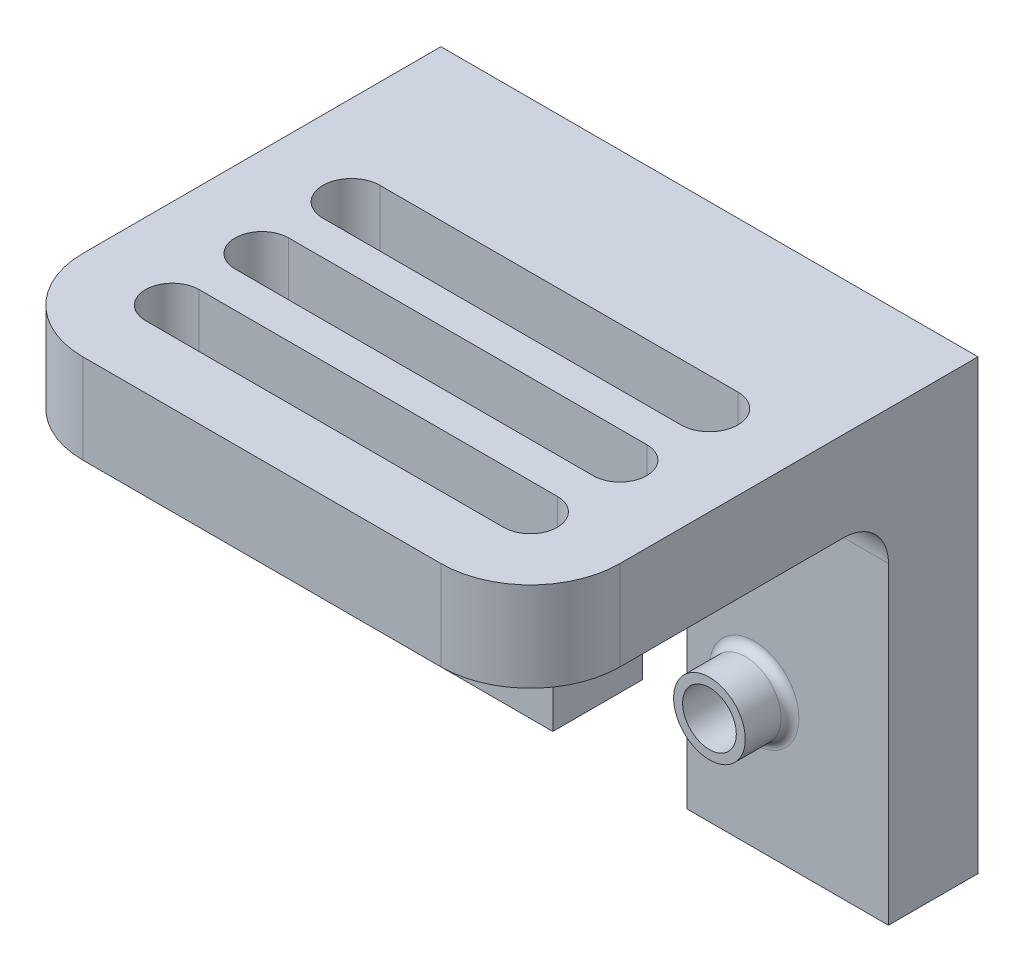
ISO-10303-21;
HEADER;
FILE_DESCRIPTION(('STEP AP214'),'2;1');
FILE_NAME('part.step','',(''),(''),'','','');
FILE_SCHEMA(('AUTOMOTIVE_DESIGN { 1 0 10303 214 1 1 1 1 }'));
ENDSEC;
DATA;
#1=APPLICATION_CONTEXT('core data for automotive mechanical design processes');
#2=APPLICATION_PROTOCOL_DEFINITION('international standard','automotive_design',2000,#1);
#3=PRODUCT_CONTEXT('',#1,'mechanical');
#4=PRODUCT('Part','Part','',(#3));
#5=PRODUCT_RELATED_PRODUCT_CATEGORY('part','',(#4));
#6=PRODUCT_DEFINITION_FORMATION('','',#4);
#7=PRODUCT_DEFINITION_CONTEXT('part definition',#1,'design');
#8=PRODUCT_DEFINITION('design','',#6,#7);
#9=PRODUCT_DEFINITION_SHAPE('','',#8);
#10=(LENGTH_UNIT() NAMED_UNIT(*) SI_UNIT(.MILLI.,.METRE.));
#11=(NAMED_UNIT(*) PLANE_ANGLE_UNIT() SI_UNIT($,.RADIAN.));
#12=(NAMED_UNIT(*) SI_UNIT($,.STERADIAN.) SOLID_ANGLE_UNIT());
#13=UNCERTAINTY_MEASURE_WITH_UNIT(LENGTH_MEASURE(1.E-05),#10,'distance_accuracy_value','');
#14=(GEOMETRIC_REPRESENTATION_CONTEXT(3) GLOBAL_UNCERTAINTY_ASSIGNED_CONTEXT((#13)) GLOBAL_UNIT_ASSIGNED_CONTEXT((#10,
#11,#12)) REPRESENTATION_CONTEXT('',''));
#15=CARTESIAN_POINT('',(0.,0.,0.));
#16=DIRECTION('',(0.,0.,1.));
#17=DIRECTION('',(1.,0.,0.));
#18=AXIS2_PLACEMENT_3D('',#15,#16,#17);
#19=CARTESIAN_POINT('',(0.,0.,20.));
#20=DIRECTION('',(0.,1.,0.));
#21=DIRECTION('',(0.,0.,1.));
#22=AXIS2_PLACEMENT_3D('',#19,#20,#21);
#23=PLANE('',#22);
#24=DIRECTION('',(1.,0.,0.));
#25=VECTOR('',#24,1.);
#26=CARTESIAN_POINT('',(0.,0.,20.));
#27=LINE('',#26,#25);
#28=CARTESIAN_POINT('',(75.,0.,20.));
#29=VERTEX_POINT('',#28);
#30=CARTESIAN_POINT('',(120.,0.,20.));
#31=VERTEX_POINT('',#30);
#32=EDGE_CURVE('E358',#29,#31,#27,.T.);
#33=ORIENTED_EDGE('',*,*,#32,.F.);
#34=DIRECTION('',(0.,0.,1.));
#35=VECTOR('',#34,1.);
#36=CARTESIAN_POINT('',(75.,0.,0.));
#37=LINE('',#36,#35);
#38=CARTESIAN_POINT('',(75.,0.,0.));
#39=VERTEX_POINT('',#38);
#40=EDGE_CURVE('E244',#39,#29,#37,.T.);
#41=ORIENTED_EDGE('',*,*,#40,.F.);
#42=DIRECTION('',(1.,0.,0.));
#43=VECTOR('',#42,1.);
#44=CARTESIAN_POINT('',(0.,0.,0.));
#45=LINE('',#44,#43);
#46=CARTESIAN_POINT('',(120.,0.,0.));
#47=VERTEX_POINT('',#46);
#48=EDGE_CURVE('E370',#39,#47,#45,.T.);
#49=ORIENTED_EDGE('',*,*,#48,.T.);
#50=DIRECTION('',(0.,0.,-1.));
#51=VECTOR('',#50,1.);
#52=CARTESIAN_POINT('',(120.,0.,20.));
#53=LINE('',#52,#51);
#54=EDGE_CURVE('E377',#31,#47,#53,.T.);
#55=ORIENTED_EDGE('',*,*,#54,.F.);
#56=EDGE_LOOP('',(#33,#41,#49,#55));
#57=FACE_BOUND('',#56,.T.);
#58=ADVANCED_FACE('F44',(#57),#23,.F.);
#59=CARTESIAN_POINT('',(0.,100.,20.));
#60=DIRECTION('',(1.,0.,0.));
#61=DIRECTION('',(0.,0.,-1.));
#62=AXIS2_PLACEMENT_3D('',#59,#60,#61);
#63=PLANE('',#62);
#64=DIRECTION('',(0.,0.,-1.));
#65=VECTOR('',#64,1.);
#66=CARTESIAN_POINT('',(0.,80.,100.));
#67=LINE('',#66,#65);
#68=CARTESIAN_POINT('',(0.,80.,80.));
#69=VERTEX_POINT('',#68);
#70=CARTESIAN_POINT('',(0.,80.,30.));
#71=VERTEX_POINT('',#70);
#72=EDGE_CURVE('E352',#69,#71,#67,.T.);
#73=ORIENTED_EDGE('',*,*,#72,.F.);
#74=DIRECTION('',(0.,-1.,0.));
#75=VECTOR('',#74,1.);
#76=CARTESIAN_POINT('',(0.,100.,80.));
#77=LINE('',#76,#75);
#78=CARTESIAN_POINT('',(0.,100.,80.));
#79=VERTEX_POINT('',#78);
#80=EDGE_CURVE('E408',#69,#79,#77,.F.);
#81=ORIENTED_EDGE('',*,*,#80,.T.);
#82=DIRECTION('',(0.,0.,-1.));
#83=VECTOR('',#82,1.);
#84=CARTESIAN_POINT('',(0.,100.,20.));
#85=LINE('',#84,#83);
#86=CARTESIAN_POINT('',(0.,100.,0.));
#87=VERTEX_POINT('',#86);
#88=EDGE_CURVE('E364',#79,#87,#85,.T.);
#89=ORIENTED_EDGE('',*,*,#88,.T.);
#90=DIRECTION('',(0.,-1.,0.));
#91=VECTOR('',#90,1.);
#92=CARTESIAN_POINT('',(0.,100.,0.));
#93=LINE('',#92,#91);
#94=CARTESIAN_POINT('',(0.,0.,0.));
#95=VERTEX_POINT('',#94);
#96=EDGE_CURVE('E354',#87,#95,#93,.T.);
#97=ORIENTED_EDGE('',*,*,#96,.T.);
#98=DIRECTION('',(0.,0.,-1.));
#99=VECTOR('',#98,1.);
#100=CARTESIAN_POINT('',(0.,0.,20.));
#101=LINE('',#100,#99);
#102=CARTESIAN_POINT('',(0.,0.,20.));
#103=VERTEX_POINT('',#102);
#104=EDGE_CURVE('E382',#103,#95,#101,.T.);
#105=ORIENTED_EDGE('',*,*,#104,.F.);
#106=DIRECTION('',(0.,-1.,0.));
#107=VECTOR('',#106,1.);
#108=CARTESIAN_POINT('',(0.,100.,20.));
#109=LINE('',#108,#107);
#110=CARTESIAN_POINT('',(0.,70.,20.));
#111=VERTEX_POINT('',#110);
#112=EDGE_CURVE('E351',#111,#103,#109,.T.);
#113=ORIENTED_EDGE('',*,*,#112,.F.);
#114=CARTESIAN_POINT('',(0.,70.,30.));
#115=DIRECTION('',(1.,0.,0.));
#116=DIRECTION('',(0.,0.,-1.));
#117=AXIS2_PLACEMENT_3D('',#114,#115,#116);
#118=CIRCLE('',#117,10.);
#119=EDGE_CURVE('E393',#111,#71,#118,.T.);
#120=ORIENTED_EDGE('',*,*,#119,.T.);
#121=EDGE_LOOP('',(#73,#81,#89,#97,#105,#113,#120));
#122=FACE_BOUND('',#121,.T.);
#123=ADVANCED_FACE('F467',(#122),#63,.F.);
#124=CARTESIAN_POINT('',(45.,0.,0.));
#125=VERTEX_POINT('',#124);
#126=EDGE_CURVE('E368',#95,#125,#45,.T.);
#127=ORIENTED_EDGE('',*,*,#126,.T.);
#128=DIRECTION('',(0.,0.,1.));
#129=VECTOR('',#128,1.);
#130=CARTESIAN_POINT('',(45.,0.,0.));
#131=LINE('',#130,#129);
#132=CARTESIAN_POINT('',(45.,0.,20.));
#133=VERTEX_POINT('',#132);
#134=EDGE_CURVE('E58',#125,#133,#131,.T.);
#135=ORIENTED_EDGE('',*,*,#134,.T.);
#136=EDGE_CURVE('E356',#103,#133,#27,.T.);
#137=ORIENTED_EDGE('',*,*,#136,.F.);
#138=ORIENTED_EDGE('',*,*,#104,.T.);
#139=EDGE_LOOP('',(#127,#135,#137,#138));
#140=FACE_BOUND('',#139,.T.);
#141=ADVANCED_FACE('F469',(#140),#23,.F.);
#142=CARTESIAN_POINT('',(120.,0.,20.));
#143=DIRECTION('',(-1.,0.,0.));
#144=DIRECTION('',(0.,0.,1.));
#145=AXIS2_PLACEMENT_3D('',#142,#143,#144);
#146=PLANE('',#145);
#147=DIRECTION('',(0.,0.,-1.));
#148=VECTOR('',#147,1.);
#149=CARTESIAN_POINT('',(120.,100.,20.));
#150=LINE('',#149,#148);
#151=CARTESIAN_POINT('',(120.,100.,80.));
#152=VERTEX_POINT('',#151);
#153=CARTESIAN_POINT('',(120.,100.,0.));
#154=VERTEX_POINT('',#153);
#155=EDGE_CURVE('E376',#152,#154,#150,.T.);
#156=ORIENTED_EDGE('',*,*,#155,.F.);
#157=DIRECTION('',(0.,1.,0.));
#158=VECTOR('',#157,1.);
#159=CARTESIAN_POINT('',(120.,80.,80.));
#160=LINE('',#159,#158);
#161=CARTESIAN_POINT('',(120.,80.,80.));
#162=VERTEX_POINT('',#161);
#163=EDGE_CURVE('E404',#152,#162,#160,.F.);
#164=ORIENTED_EDGE('',*,*,#163,.T.);
#165=DIRECTION('',(0.,0.,-1.));
#166=VECTOR('',#165,1.);
#167=CARTESIAN_POINT('',(120.,80.,100.));
#168=LINE('',#167,#166);
#169=CARTESIAN_POINT('',(120.,80.,30.));
#170=VERTEX_POINT('',#169);
#171=EDGE_CURVE('E350',#162,#170,#168,.T.);
#172=ORIENTED_EDGE('',*,*,#171,.T.);
#173=CARTESIAN_POINT('',(120.,70.,30.));
#174=DIRECTION('',(-1.,0.,0.));
#175=DIRECTION('',(0.,0.,1.));
#176=AXIS2_PLACEMENT_3D('',#173,#174,#175);
#177=CIRCLE('',#176,10.);
#178=CARTESIAN_POINT('',(120.,70.,20.));
#179=VERTEX_POINT('',#178);
#180=EDGE_CURVE('E388',#170,#179,#177,.T.);
#181=ORIENTED_EDGE('',*,*,#180,.T.);
#182=DIRECTION('',(0.,1.,0.));
#183=VECTOR('',#182,1.);
#184=CARTESIAN_POINT('',(120.,0.,20.));
#185=LINE('',#184,#183);
#186=EDGE_CURVE('E363',#31,#179,#185,.T.);
#187=ORIENTED_EDGE('',*,*,#186,.F.);
#188=ORIENTED_EDGE('',*,*,#54,.T.);
#189=DIRECTION('',(0.,1.,0.));
#190=VECTOR('',#189,1.);
#191=CARTESIAN_POINT('',(120.,0.,0.));
#192=LINE('',#191,#190);
#193=EDGE_CURVE('E369',#47,#154,#192,.T.);
#194=ORIENTED_EDGE('',*,*,#193,.T.);
#195=EDGE_LOOP('',(#156,#164,#172,#181,#187,#188,#194));
#196=FACE_BOUND('',#195,.T.);
#197=ADVANCED_FACE('F480',(#196),#146,.F.);
#198=CARTESIAN_POINT('',(120.,100.,20.));
#199=DIRECTION('',(0.,-1.,0.));
#200=DIRECTION('',(0.,0.,-1.));
#201=AXIS2_PLACEMENT_3D('',#198,#199,#200);
#202=PLANE('',#201);
#203=DIRECTION('',(-1.,0.,0.));
#204=VECTOR('',#203,1.);
#205=CARTESIAN_POINT('',(20.,100.,46.3648555008302));
#206=LINE('',#205,#204);
#207=CARTESIAN_POINT('',(100.,100.,46.3648555008302));
#208=VERTEX_POINT('',#207);
#209=CARTESIAN_POINT('',(20.,100.,46.3648555008302));
#210=VERTEX_POINT('',#209);
#211=EDGE_CURVE('E260',#208,#210,#206,.T.);
#212=ORIENTED_EDGE('',*,*,#211,.T.);
#213=CARTESIAN_POINT('',(20.,100.,40.));
#214=DIRECTION('',(0.,-1.,0.));
#215=DIRECTION('',(0.,0.,-1.));
#216=AXIS2_PLACEMENT_3D('',#213,#214,#215);
#217=CIRCLE('',#216,6.36485550083021);
#218=CARTESIAN_POINT('',(20.,100.,33.6351444991698));
#219=VERTEX_POINT('',#218);
#220=EDGE_CURVE('E247',#210,#219,#217,.T.);
#221=ORIENTED_EDGE('',*,*,#220,.T.);
#222=DIRECTION('',(1.,0.,0.));
#223=VECTOR('',#222,1.);
#224=CARTESIAN_POINT('',(20.,100.,33.6351444991698));
#225=LINE('',#224,#223);
#226=CARTESIAN_POINT('',(100.,100.,33.6351444991698));
#227=VERTEX_POINT('',#226);
#228=EDGE_CURVE('E252',#219,#227,#225,.T.);
#229=ORIENTED_EDGE('',*,*,#228,.T.);
#230=CARTESIAN_POINT('',(100.,100.,40.));
#231=DIRECTION('',(0.,-1.,0.));
#232=DIRECTION('',(0.,0.,-1.));
#233=AXIS2_PLACEMENT_3D('',#230,#231,#232);
#234=CIRCLE('',#233,6.36485550083021);
#235=EDGE_CURVE('E253',#227,#208,#234,.T.);
#236=ORIENTED_EDGE('',*,*,#235,.T.);
#237=EDGE_LOOP('',(#212,#221,#229,#236));
#238=FACE_BOUND('',#237,.T.);
#239=DIRECTION('',(-1.,0.,0.));
#240=VECTOR('',#239,1.);
#241=CARTESIAN_POINT('',(20.,100.,66.));
#242=LINE('',#241,#240);
#243=CARTESIAN_POINT('',(100.,100.,66.));
#244=VERTEX_POINT('',#243);
#245=CARTESIAN_POINT('',(20.,100.,66.));
#246=VERTEX_POINT('',#245);
#247=EDGE_CURVE('E288',#244,#246,#242,.T.);
#248=ORIENTED_EDGE('',*,*,#247,.T.);
#249=CARTESIAN_POINT('',(20.,100.,60.));
#250=DIRECTION('',(0.,-1.,0.));
#251=DIRECTION('',(0.,0.,-1.));
#252=AXIS2_PLACEMENT_3D('',#249,#250,#251);
#253=CIRCLE('',#252,6.00000000000001);
#254=CARTESIAN_POINT('',(20.,100.,54.));
#255=VERTEX_POINT('',#254);
#256=EDGE_CURVE('E277',#246,#255,#253,.T.);
#257=ORIENTED_EDGE('',*,*,#256,.T.);
#258=DIRECTION('',(1.,0.,0.));
#259=VECTOR('',#258,1.);
#260=CARTESIAN_POINT('',(20.,100.,54.));
#261=LINE('',#260,#259);
#262=CARTESIAN_POINT('',(100.,100.,54.));
#263=VERTEX_POINT('',#262);
#264=EDGE_CURVE('E282',#255,#263,#261,.T.);
#265=ORIENTED_EDGE('',*,*,#264,.T.);
#266=CARTESIAN_POINT('',(100.,100.,60.));
#267=DIRECTION('',(0.,-1.,0.));
#268=DIRECTION('',(0.,0.,-1.));
#269=AXIS2_PLACEMENT_3D('',#266,#267,#268);
#270=CIRCLE('',#269,6.00000000000001);
#271=EDGE_CURVE('E290',#263,#244,#270,.T.);
#272=ORIENTED_EDGE('',*,*,#271,.T.);
#273=EDGE_LOOP('',(#248,#257,#265,#272));
#274=FACE_BOUND('',#273,.T.);
#275=DIRECTION('',(-1.,0.,0.));
#276=VECTOR('',#275,1.);
#277=CARTESIAN_POINT('',(20.,100.,86.));
#278=LINE('',#277,#276);
#279=CARTESIAN_POINT('',(100.,100.,86.));
#280=VERTEX_POINT('',#279);
#281=CARTESIAN_POINT('',(20.,100.,86.));
#282=VERTEX_POINT('',#281);
#283=EDGE_CURVE('E321',#280,#282,#278,.T.);
#284=ORIENTED_EDGE('',*,*,#283,.T.);
#285=CARTESIAN_POINT('',(20.,100.,80.));
#286=DIRECTION('',(0.,-1.,0.));
#287=DIRECTION('',(0.,0.,-1.));
#288=AXIS2_PLACEMENT_3D('',#285,#286,#287);
#289=CIRCLE('',#288,6.00000000000001);
#290=CARTESIAN_POINT('',(20.,100.,74.));
#291=VERTEX_POINT('',#290);
#292=EDGE_CURVE('E315',#282,#291,#289,.T.);
#293=ORIENTED_EDGE('',*,*,#292,.T.);
#294=DIRECTION('',(1.,0.,0.));
#295=VECTOR('',#294,1.);
#296=CARTESIAN_POINT('',(20.,100.,74.));
#297=LINE('',#296,#295);
#298=CARTESIAN_POINT('',(100.,100.,74.));
#299=VERTEX_POINT('',#298);
#300=EDGE_CURVE('E314',#291,#299,#297,.T.);
#301=ORIENTED_EDGE('',*,*,#300,.T.);
#302=CARTESIAN_POINT('',(100.,100.,80.));
#303=DIRECTION('',(0.,-1.,0.));
#304=DIRECTION('',(0.,0.,-1.));
#305=AXIS2_PLACEMENT_3D('',#302,#303,#304);
#306=CIRCLE('',#305,6.00000000000001);
#307=EDGE_CURVE('E316',#299,#280,#306,.T.);
#308=ORIENTED_EDGE('',*,*,#307,.T.);
#309=EDGE_LOOP('',(#284,#293,#301,#308));
#310=FACE_BOUND('',#309,.T.);
#311=DIRECTION('',(-1.,0.,0.));
#312=VECTOR('',#311,1.);
#313=CARTESIAN_POINT('',(0.,100.,100.));
#314=LINE('',#313,#312);
#315=CARTESIAN_POINT('',(100.,100.,100.));
#316=VERTEX_POINT('',#315);
#317=CARTESIAN_POINT('',(20.,100.,100.));
#318=VERTEX_POINT('',#317);
#319=EDGE_CURVE('E348',#316,#318,#314,.T.);
#320=ORIENTED_EDGE('',*,*,#319,.F.);
#321=CARTESIAN_POINT('',(100.,100.,80.));
#322=DIRECTION('',(0.,-1.,0.));
#323=DIRECTION('',(0.,0.,-1.));
#324=AXIS2_PLACEMENT_3D('',#321,#322,#323);
#325=CIRCLE('',#324,20.);
#326=EDGE_CURVE('E405',#316,#152,#325,.F.);
#327=ORIENTED_EDGE('',*,*,#326,.T.);
#328=ORIENTED_EDGE('',*,*,#155,.T.);
#329=DIRECTION('',(-1.,0.,0.));
#330=VECTOR('',#329,1.);
#331=CARTESIAN_POINT('',(120.,100.,0.));
#332=LINE('',#331,#330);
#333=EDGE_CURVE('E357',#154,#87,#332,.T.);
#334=ORIENTED_EDGE('',*,*,#333,.T.);
#335=ORIENTED_EDGE('',*,*,#88,.F.);
#336=CARTESIAN_POINT('',(20.,100.,80.));
#337=DIRECTION('',(0.,-1.,0.));
#338=DIRECTION('',(0.,0.,-1.));
#339=AXIS2_PLACEMENT_3D('',#336,#337,#338);
#340=CIRCLE('',#339,20.);
#341=EDGE_CURVE('E398',#79,#318,#340,.F.);
#342=ORIENTED_EDGE('',*,*,#341,.T.);
#343=EDGE_LOOP('',(#320,#327,#328,#334,#335,#342));
#344=FACE_BOUND('',#343,.T.);
#345=ADVANCED_FACE('F483',(#238,#274,#310,#344),#202,.F.);
#346=CARTESIAN_POINT('',(0.,0.,20.));
#347=DIRECTION('',(0.,0.,1.));
#348=DIRECTION('',(1.,0.,0.));
#349=AXIS2_PLACEMENT_3D('',#346,#347,#348);
#350=PLANE('',#349);
#351=CARTESIAN_POINT('',(90.,30.,20.));
#352=DIRECTION('',(0.,0.,1.));
#353=DIRECTION('',(1.,0.,0.));
#354=AXIS2_PLACEMENT_3D('',#351,#352,#353);
#355=CIRCLE('',#354,10.);
#356=CARTESIAN_POINT('',(100.,30.,20.));
#357=VERTEX_POINT('',#356);
#358=EDGE_CURVE('E52',#357,#357,#355,.F.);
#359=ORIENTED_EDGE('',*,*,#358,.T.);
#360=EDGE_LOOP('',(#359));
#361=FACE_BOUND('',#360,.T.);
#362=CARTESIAN_POINT('',(30.,30.,20.));
#363=DIRECTION('',(0.,0.,1.));
#364=DIRECTION('',(1.,0.,0.));
#365=AXIS2_PLACEMENT_3D('',#362,#363,#364);
#366=CIRCLE('',#365,10.);
#367=CARTESIAN_POINT('',(40.,30.,20.));
#368=VERTEX_POINT('',#367);
#369=EDGE_CURVE('E418',#368,#368,#366,.F.);
#370=ORIENTED_EDGE('',*,*,#369,.T.);
#371=EDGE_LOOP('',(#370));
#372=FACE_BOUND('',#371,.T.);
#373=DIRECTION('',(0.,1.,0.));
#374=VECTOR('',#373,1.);
#375=CARTESIAN_POINT('',(75.,0.,20.));
#376=LINE('',#375,#374);
#377=CARTESIAN_POINT('',(75.,35.,20.));
#378=VERTEX_POINT('',#377);
#379=EDGE_CURVE('E229',#29,#378,#376,.T.);
#380=ORIENTED_EDGE('',*,*,#379,.F.);
#381=ORIENTED_EDGE('',*,*,#32,.T.);
#382=ORIENTED_EDGE('',*,*,#186,.T.);
#383=DIRECTION('',(1.,0.,0.));
#384=VECTOR('',#383,1.);
#385=CARTESIAN_POINT('',(0.,70.,20.));
#386=LINE('',#385,#384);
#387=EDGE_CURVE('E386',#179,#111,#386,.F.);
#388=ORIENTED_EDGE('',*,*,#387,.T.);
#389=ORIENTED_EDGE('',*,*,#112,.T.);
#390=ORIENTED_EDGE('',*,*,#136,.T.);
#391=DIRECTION('',(0.,-1.,0.));
#392=VECTOR('',#391,1.);
#393=CARTESIAN_POINT('',(45.,35.,20.));
#394=LINE('',#393,#392);
#395=CARTESIAN_POINT('',(45.,35.,20.));
#396=VERTEX_POINT('',#395);
#397=EDGE_CURVE('E231',#396,#133,#394,.T.);
#398=ORIENTED_EDGE('',*,*,#397,.F.);
#399=CARTESIAN_POINT('',(60.,35.,20.));
#400=DIRECTION('',(0.,0.,1.));
#401=DIRECTION('',(1.,0.,0.));
#402=AXIS2_PLACEMENT_3D('',#399,#400,#401);
#403=CIRCLE('',#402,15.);
#404=EDGE_CURVE('E220',#378,#396,#403,.T.);
#405=ORIENTED_EDGE('',*,*,#404,.F.);
#406=EDGE_LOOP('',(#380,#381,#382,#388,#389,#390,#398,#405));
#407=FACE_BOUND('',#406,.T.);
#408=ADVANCED_FACE('F424',(#361,#372,#407),#350,.T.);
#409=CARTESIAN_POINT('',(0.,0.,0.));
#410=DIRECTION('',(0.,0.,1.));
#411=DIRECTION('',(1.,0.,0.));
#412=AXIS2_PLACEMENT_3D('',#409,#410,#411);
#413=PLANE('',#412);
#414=ORIENTED_EDGE('',*,*,#48,.F.);
#415=DIRECTION('',(0.,1.,0.));
#416=VECTOR('',#415,1.);
#417=CARTESIAN_POINT('',(75.,0.,0.));
#418=LINE('',#417,#416);
#419=CARTESIAN_POINT('',(75.,35.,0.));
#420=VERTEX_POINT('',#419);
#421=EDGE_CURVE('E222',#39,#420,#418,.T.);
#422=ORIENTED_EDGE('',*,*,#421,.T.);
#423=CARTESIAN_POINT('',(60.,35.,0.));
#424=DIRECTION('',(0.,0.,1.));
#425=DIRECTION('',(1.,0.,0.));
#426=AXIS2_PLACEMENT_3D('',#423,#424,#425);
#427=CIRCLE('',#426,15.);
#428=CARTESIAN_POINT('',(45.,35.,0.));
#429=VERTEX_POINT('',#428);
#430=EDGE_CURVE('E218',#420,#429,#427,.T.);
#431=ORIENTED_EDGE('',*,*,#430,.T.);
#432=DIRECTION('',(0.,-1.,0.));
#433=VECTOR('',#432,1.);
#434=CARTESIAN_POINT('',(45.,35.,0.));
#435=LINE('',#434,#433);
#436=EDGE_CURVE('E224',#429,#125,#435,.T.);
#437=ORIENTED_EDGE('',*,*,#436,.T.);
#438=ORIENTED_EDGE('',*,*,#126,.F.);
#439=ORIENTED_EDGE('',*,*,#96,.F.);
#440=ORIENTED_EDGE('',*,*,#333,.F.);
#441=ORIENTED_EDGE('',*,*,#193,.F.);
#442=EDGE_LOOP('',(#414,#422,#431,#437,#438,#439,#440,#441));
#443=FACE_BOUND('',#442,.T.);
#444=ADVANCED_FACE('F230',(#443),#413,.F.);
#445=CARTESIAN_POINT('',(0.,80.,100.));
#446=DIRECTION('',(0.,1.,0.));
#447=DIRECTION('',(0.,0.,1.));
#448=AXIS2_PLACEMENT_3D('',#445,#446,#447);
#449=PLANE('',#448);
#450=DIRECTION('',(1.,0.,0.));
#451=VECTOR('',#450,1.);
#452=CARTESIAN_POINT('',(20.,80.,33.6351444991698));
#453=LINE('',#452,#451);
#454=CARTESIAN_POINT('',(20.,80.,33.6351444991698));
#455=VERTEX_POINT('',#454);
#456=CARTESIAN_POINT('',(100.,80.,33.6351444991698));
#457=VERTEX_POINT('',#456);
#458=EDGE_CURVE('E262',#455,#457,#453,.T.);
#459=ORIENTED_EDGE('',*,*,#458,.F.);
#460=CARTESIAN_POINT('',(20.,80.,40.));
#461=DIRECTION('',(0.,-1.,0.));
#462=DIRECTION('',(0.,0.,-1.));
#463=AXIS2_PLACEMENT_3D('',#460,#461,#462);
#464=CIRCLE('',#463,6.36485550083021);
#465=CARTESIAN_POINT('',(20.,80.,46.3648555008302));
#466=VERTEX_POINT('',#465);
#467=EDGE_CURVE('E242',#466,#455,#464,.T.);
#468=ORIENTED_EDGE('',*,*,#467,.F.);
#469=DIRECTION('',(-1.,0.,0.));
#470=VECTOR('',#469,1.);
#471=CARTESIAN_POINT('',(20.,80.,46.3648555008302));
#472=LINE('',#471,#470);
#473=CARTESIAN_POINT('',(100.,80.,46.3648555008302));
#474=VERTEX_POINT('',#473);
#475=EDGE_CURVE('E255',#474,#466,#472,.T.);
#476=ORIENTED_EDGE('',*,*,#475,.F.);
#477=CARTESIAN_POINT('',(100.,80.,40.));
#478=DIRECTION('',(0.,-1.,0.));
#479=DIRECTION('',(0.,0.,-1.));
#480=AXIS2_PLACEMENT_3D('',#477,#478,#479);
#481=CIRCLE('',#480,6.36485550083021);
#482=EDGE_CURVE('E267',#457,#474,#481,.T.);
#483=ORIENTED_EDGE('',*,*,#482,.F.);
#484=EDGE_LOOP('',(#459,#468,#476,#483));
#485=FACE_BOUND('',#484,.T.);
#486=DIRECTION('',(1.,0.,0.));
#487=VECTOR('',#486,1.);
#488=CARTESIAN_POINT('',(20.,80.,54.));
#489=LINE('',#488,#487);
#490=CARTESIAN_POINT('',(20.,80.,54.));
#491=VERTEX_POINT('',#490);
#492=CARTESIAN_POINT('',(100.,80.,54.));
#493=VERTEX_POINT('',#492);
#494=EDGE_CURVE('E294',#491,#493,#489,.T.);
#495=ORIENTED_EDGE('',*,*,#494,.F.);
#496=CARTESIAN_POINT('',(20.,80.,60.));
#497=DIRECTION('',(0.,-1.,0.));
#498=DIRECTION('',(0.,0.,-1.));
#499=AXIS2_PLACEMENT_3D('',#496,#497,#498);
#500=CIRCLE('',#499,6.00000000000001);
#501=CARTESIAN_POINT('',(20.,80.,66.));
#502=VERTEX_POINT('',#501);
#503=EDGE_CURVE('E271',#502,#491,#500,.T.);
#504=ORIENTED_EDGE('',*,*,#503,.F.);
#505=DIRECTION('',(-1.,0.,0.));
#506=VECTOR('',#505,1.);
#507=CARTESIAN_POINT('',(20.,80.,66.));
#508=LINE('',#507,#506);
#509=CARTESIAN_POINT('',(100.,80.,66.));
#510=VERTEX_POINT('',#509);
#511=EDGE_CURVE('E285',#510,#502,#508,.T.);
#512=ORIENTED_EDGE('',*,*,#511,.F.);
#513=CARTESIAN_POINT('',(100.,80.,60.));
#514=DIRECTION('',(0.,-1.,0.));
#515=DIRECTION('',(0.,0.,-1.));
#516=AXIS2_PLACEMENT_3D('',#513,#514,#515);
#517=CIRCLE('',#516,6.00000000000001);
#518=EDGE_CURVE('E296',#493,#510,#517,.T.);
#519=ORIENTED_EDGE('',*,*,#518,.F.);
#520=EDGE_LOOP('',(#495,#504,#512,#519));
#521=FACE_BOUND('',#520,.T.);
#522=DIRECTION('',(1.,0.,0.));
#523=VECTOR('',#522,1.);
#524=CARTESIAN_POINT('',(20.,80.,74.));
#525=LINE('',#524,#523);
#526=CARTESIAN_POINT('',(20.,80.,74.));
#527=VERTEX_POINT('',#526);
#528=CARTESIAN_POINT('',(100.,80.,74.));
#529=VERTEX_POINT('',#528);
#530=EDGE_CURVE('E329',#527,#529,#525,.T.);
#531=ORIENTED_EDGE('',*,*,#530,.F.);
#532=CARTESIAN_POINT('',(20.,80.,80.));
#533=DIRECTION('',(0.,-1.,0.));
#534=DIRECTION('',(0.,0.,-1.));
#535=AXIS2_PLACEMENT_3D('',#532,#533,#534);
#536=CIRCLE('',#535,6.00000000000001);
#537=CARTESIAN_POINT('',(20.,80.,86.));
#538=VERTEX_POINT('',#537);
#539=EDGE_CURVE('E304',#538,#527,#536,.T.);
#540=ORIENTED_EDGE('',*,*,#539,.F.);
#541=DIRECTION('',(-1.,0.,0.));
#542=VECTOR('',#541,1.);
#543=CARTESIAN_POINT('',(20.,80.,86.));
#544=LINE('',#543,#542);
#545=CARTESIAN_POINT('',(100.,80.,86.));
#546=VERTEX_POINT('',#545);
#547=EDGE_CURVE('E317',#546,#538,#544,.T.);
#548=ORIENTED_EDGE('',*,*,#547,.F.);
#549=CARTESIAN_POINT('',(100.,80.,80.));
#550=DIRECTION('',(0.,-1.,0.));
#551=DIRECTION('',(0.,0.,-1.));
#552=AXIS2_PLACEMENT_3D('',#549,#550,#551);
#553=CIRCLE('',#552,6.00000000000001);
#554=EDGE_CURVE('E326',#529,#546,#553,.T.);
#555=ORIENTED_EDGE('',*,*,#554,.F.);
#556=EDGE_LOOP('',(#531,#540,#548,#555));
#557=FACE_BOUND('',#556,.T.);
#558=ORIENTED_EDGE('',*,*,#171,.F.);
#559=CARTESIAN_POINT('',(100.,80.,80.));
#560=DIRECTION('',(0.,1.,0.));
#561=DIRECTION('',(0.,0.,1.));
#562=AXIS2_PLACEMENT_3D('',#559,#560,#561);
#563=CIRCLE('',#562,20.);
#564=CARTESIAN_POINT('',(100.,80.,100.));
#565=VERTEX_POINT('',#564);
#566=EDGE_CURVE('E406',#162,#565,#563,.F.);
#567=ORIENTED_EDGE('',*,*,#566,.T.);
#568=DIRECTION('',(1.,0.,0.));
#569=VECTOR('',#568,1.);
#570=CARTESIAN_POINT('',(0.,80.,100.));
#571=LINE('',#570,#569);
#572=CARTESIAN_POINT('',(20.,80.,100.));
#573=VERTEX_POINT('',#572);
#574=EDGE_CURVE('E340',#573,#565,#571,.T.);
#575=ORIENTED_EDGE('',*,*,#574,.F.);
#576=CARTESIAN_POINT('',(20.,80.,80.));
#577=DIRECTION('',(0.,1.,0.));
#578=DIRECTION('',(0.,0.,1.));
#579=AXIS2_PLACEMENT_3D('',#576,#577,#578);
#580=CIRCLE('',#579,20.);
#581=EDGE_CURVE('E67',#573,#69,#580,.F.);
#582=ORIENTED_EDGE('',*,*,#581,.T.);
#583=ORIENTED_EDGE('',*,*,#72,.T.);
#584=DIRECTION('',(1.,0.,0.));
#585=VECTOR('',#584,1.);
#586=CARTESIAN_POINT('',(0.,80.,30.));
#587=LINE('',#586,#585);
#588=EDGE_CURVE('E381',#71,#170,#587,.T.);
#589=ORIENTED_EDGE('',*,*,#588,.T.);
#590=EDGE_LOOP('',(#558,#567,#575,#582,#583,#589));
#591=FACE_BOUND('',#590,.T.);
#592=ADVANCED_FACE('F511',(#485,#521,#557,#591),#449,.F.);
#593=CARTESIAN_POINT('',(0.,0.,100.));
#594=DIRECTION('',(0.,0.,1.));
#595=DIRECTION('',(1.,0.,0.));
#596=AXIS2_PLACEMENT_3D('',#593,#594,#595);
#597=PLANE('',#596);
#598=ORIENTED_EDGE('',*,*,#574,.T.);
#599=DIRECTION('',(0.,1.,0.));
#600=VECTOR('',#599,1.);
#601=CARTESIAN_POINT('',(100.,100.,100.));
#602=LINE('',#601,#600);
#603=EDGE_CURVE('E400',#565,#316,#602,.T.);
#604=ORIENTED_EDGE('',*,*,#603,.T.);
#605=ORIENTED_EDGE('',*,*,#319,.T.);
#606=DIRECTION('',(0.,-1.,0.));
#607=VECTOR('',#606,1.);
#608=CARTESIAN_POINT('',(20.,80.,100.));
#609=LINE('',#608,#607);
#610=EDGE_CURVE('E395',#318,#573,#609,.T.);
#611=ORIENTED_EDGE('',*,*,#610,.T.);
#612=EDGE_LOOP('',(#598,#604,#605,#611));
#613=FACE_BOUND('',#612,.T.);
#614=ADVANCED_FACE('F517',(#613),#597,.T.);
#615=CARTESIAN_POINT('',(20.,100.,80.));
#616=DIRECTION('',(0.,-1.,0.));
#617=DIRECTION('',(0.,0.,-1.));
#618=AXIS2_PLACEMENT_3D('',#615,#616,#617);
#619=CYLINDRICAL_SURFACE('',#618,6.00000000000001);
#620=ORIENTED_EDGE('',*,*,#539,.T.);
#621=DIRECTION('',(0.,-1.,0.));
#622=VECTOR('',#621,1.);
#623=CARTESIAN_POINT('',(20.,100.,74.));
#624=LINE('',#623,#622);
#625=EDGE_CURVE('E322',#291,#527,#624,.T.);
#626=ORIENTED_EDGE('',*,*,#625,.F.);
#627=ORIENTED_EDGE('',*,*,#292,.F.);
#628=DIRECTION('',(0.,-1.,0.));
#629=VECTOR('',#628,1.);
#630=CARTESIAN_POINT('',(20.,100.,86.));
#631=LINE('',#630,#629);
#632=EDGE_CURVE('E333',#282,#538,#631,.T.);
#633=ORIENTED_EDGE('',*,*,#632,.T.);
#634=EDGE_LOOP('',(#620,#626,#627,#633));
#635=FACE_BOUND('',#634,.T.);
#636=ADVANCED_FACE('F572',(#635),#619,.F.);
#637=CARTESIAN_POINT('',(20.,100.,86.));
#638=DIRECTION('',(0.,0.,1.));
#639=DIRECTION('',(1.,0.,0.));
#640=AXIS2_PLACEMENT_3D('',#637,#638,#639);
#641=PLANE('',#640);
#642=ORIENTED_EDGE('',*,*,#547,.T.);
#643=ORIENTED_EDGE('',*,*,#632,.F.);
#644=ORIENTED_EDGE('',*,*,#283,.F.);
#645=DIRECTION('',(0.,-1.,0.));
#646=VECTOR('',#645,1.);
#647=CARTESIAN_POINT('',(100.,100.,86.));
#648=LINE('',#647,#646);
#649=EDGE_CURVE('E336',#280,#546,#648,.T.);
#650=ORIENTED_EDGE('',*,*,#649,.T.);
#651=EDGE_LOOP('',(#642,#643,#644,#650));
#652=FACE_BOUND('',#651,.T.);
#653=ADVANCED_FACE('F567',(#652),#641,.F.);
#654=CARTESIAN_POINT('',(100.,100.,80.));
#655=DIRECTION('',(0.,-1.,0.));
#656=DIRECTION('',(0.,0.,-1.));
#657=AXIS2_PLACEMENT_3D('',#654,#655,#656);
#658=CYLINDRICAL_SURFACE('',#657,6.00000000000001);
#659=ORIENTED_EDGE('',*,*,#554,.T.);
#660=ORIENTED_EDGE('',*,*,#649,.F.);
#661=ORIENTED_EDGE('',*,*,#307,.F.);
#662=DIRECTION('',(0.,-1.,0.));
#663=VECTOR('',#662,1.);
#664=CARTESIAN_POINT('',(100.,100.,74.));
#665=LINE('',#664,#663);
#666=EDGE_CURVE('E338',#299,#529,#665,.T.);
#667=ORIENTED_EDGE('',*,*,#666,.T.);
#668=EDGE_LOOP('',(#659,#660,#661,#667));
#669=FACE_BOUND('',#668,.T.);
#670=ADVANCED_FACE('F575',(#669),#658,.F.);
#671=CARTESIAN_POINT('',(20.,100.,74.));
#672=DIRECTION('',(0.,0.,-1.));
#673=DIRECTION('',(-1.,0.,0.));
#674=AXIS2_PLACEMENT_3D('',#671,#672,#673);
#675=PLANE('',#674);
#676=ORIENTED_EDGE('',*,*,#530,.T.);
#677=ORIENTED_EDGE('',*,*,#666,.F.);
#678=ORIENTED_EDGE('',*,*,#300,.F.);
#679=ORIENTED_EDGE('',*,*,#625,.T.);
#680=EDGE_LOOP('',(#676,#677,#678,#679));
#681=FACE_BOUND('',#680,.T.);
#682=ADVANCED_FACE('F570',(#681),#675,.F.);
#683=CARTESIAN_POINT('',(20.,100.,60.));
#684=DIRECTION('',(0.,-1.,0.));
#685=DIRECTION('',(0.,0.,-1.));
#686=AXIS2_PLACEMENT_3D('',#683,#684,#685);
#687=CYLINDRICAL_SURFACE('',#686,6.00000000000001);
#688=ORIENTED_EDGE('',*,*,#503,.T.);
#689=DIRECTION('',(0.,-1.,0.));
#690=VECTOR('',#689,1.);
#691=CARTESIAN_POINT('',(20.,100.,54.));
#692=LINE('',#691,#690);
#693=EDGE_CURVE('E291',#255,#491,#692,.T.);
#694=ORIENTED_EDGE('',*,*,#693,.F.);
#695=ORIENTED_EDGE('',*,*,#256,.F.);
#696=DIRECTION('',(0.,-1.,0.));
#697=VECTOR('',#696,1.);
#698=CARTESIAN_POINT('',(20.,100.,66.));
#699=LINE('',#698,#697);
#700=EDGE_CURVE('E303',#246,#502,#699,.T.);
#701=ORIENTED_EDGE('',*,*,#700,.T.);
#702=EDGE_LOOP('',(#688,#694,#695,#701));
#703=FACE_BOUND('',#702,.T.);
#704=ADVANCED_FACE('F560',(#703),#687,.F.);
#705=CARTESIAN_POINT('',(20.,100.,66.));
#706=DIRECTION('',(0.,0.,1.));
#707=DIRECTION('',(1.,0.,0.));
#708=AXIS2_PLACEMENT_3D('',#705,#706,#707);
#709=PLANE('',#708);
#710=ORIENTED_EDGE('',*,*,#511,.T.);
#711=ORIENTED_EDGE('',*,*,#700,.F.);
#712=ORIENTED_EDGE('',*,*,#247,.F.);
#713=DIRECTION('',(0.,-1.,0.));
#714=VECTOR('',#713,1.);
#715=CARTESIAN_POINT('',(100.,100.,66.));
#716=LINE('',#715,#714);
#717=EDGE_CURVE('E306',#244,#510,#716,.T.);
#718=ORIENTED_EDGE('',*,*,#717,.T.);
#719=EDGE_LOOP('',(#710,#711,#712,#718));
#720=FACE_BOUND('',#719,.T.);
#721=ADVANCED_FACE('F551',(#720),#709,.F.);
#722=CARTESIAN_POINT('',(100.,100.,60.));
#723=DIRECTION('',(0.,-1.,0.));
#724=DIRECTION('',(0.,0.,-1.));
#725=AXIS2_PLACEMENT_3D('',#722,#723,#724);
#726=CYLINDRICAL_SURFACE('',#725,6.00000000000001);
#727=ORIENTED_EDGE('',*,*,#518,.T.);
#728=ORIENTED_EDGE('',*,*,#717,.F.);
#729=ORIENTED_EDGE('',*,*,#271,.F.);
#730=DIRECTION('',(0.,-1.,0.));
#731=VECTOR('',#730,1.);
#732=CARTESIAN_POINT('',(100.,100.,54.));
#733=LINE('',#732,#731);
#734=EDGE_CURVE('E308',#263,#493,#733,.T.);
#735=ORIENTED_EDGE('',*,*,#734,.T.);
#736=EDGE_LOOP('',(#727,#728,#729,#735));
#737=FACE_BOUND('',#736,.T.);
#738=ADVANCED_FACE('F558',(#737),#726,.F.);
#739=CARTESIAN_POINT('',(20.,100.,54.));
#740=DIRECTION('',(0.,0.,-1.));
#741=DIRECTION('',(-1.,0.,0.));
#742=AXIS2_PLACEMENT_3D('',#739,#740,#741);
#743=PLANE('',#742);
#744=ORIENTED_EDGE('',*,*,#494,.T.);
#745=ORIENTED_EDGE('',*,*,#734,.F.);
#746=ORIENTED_EDGE('',*,*,#264,.F.);
#747=ORIENTED_EDGE('',*,*,#693,.T.);
#748=EDGE_LOOP('',(#744,#745,#746,#747));
#749=FACE_BOUND('',#748,.T.);
#750=ADVANCED_FACE('F553',(#749),#743,.F.);
#751=CARTESIAN_POINT('',(20.,100.,40.));
#752=DIRECTION('',(0.,-1.,0.));
#753=DIRECTION('',(0.,0.,-1.));
#754=AXIS2_PLACEMENT_3D('',#751,#752,#753);
#755=CYLINDRICAL_SURFACE('',#754,6.36485550083021);
#756=ORIENTED_EDGE('',*,*,#467,.T.);
#757=DIRECTION('',(0.,-1.,0.));
#758=VECTOR('',#757,1.);
#759=CARTESIAN_POINT('',(20.,100.,33.6351444991698));
#760=LINE('',#759,#758);
#761=EDGE_CURVE('E263',#219,#455,#760,.T.);
#762=ORIENTED_EDGE('',*,*,#761,.F.);
#763=ORIENTED_EDGE('',*,*,#220,.F.);
#764=DIRECTION('',(0.,-1.,0.));
#765=VECTOR('',#764,1.);
#766=CARTESIAN_POINT('',(20.,100.,46.3648555008302));
#767=LINE('',#766,#765);
#768=EDGE_CURVE('E272',#210,#466,#767,.T.);
#769=ORIENTED_EDGE('',*,*,#768,.T.);
#770=EDGE_LOOP('',(#756,#762,#763,#769));
#771=FACE_BOUND('',#770,.T.);
#772=ADVANCED_FACE('F549',(#771),#755,.F.);
#773=CARTESIAN_POINT('',(20.,100.,46.3648555008302));
#774=DIRECTION('',(0.,0.,1.));
#775=DIRECTION('',(1.,0.,0.));
#776=AXIS2_PLACEMENT_3D('',#773,#774,#775);
#777=PLANE('',#776);
#778=ORIENTED_EDGE('',*,*,#475,.T.);
#779=ORIENTED_EDGE('',*,*,#768,.F.);
#780=ORIENTED_EDGE('',*,*,#211,.F.);
#781=DIRECTION('',(0.,-1.,0.));
#782=VECTOR('',#781,1.);
#783=CARTESIAN_POINT('',(100.,100.,46.3648555008302));
#784=LINE('',#783,#782);
#785=EDGE_CURVE('E274',#208,#474,#784,.T.);
#786=ORIENTED_EDGE('',*,*,#785,.T.);
#787=EDGE_LOOP('',(#778,#779,#780,#786));
#788=FACE_BOUND('',#787,.T.);
#789=ADVANCED_FACE('F542',(#788),#777,.F.);
#790=CARTESIAN_POINT('',(100.,100.,40.));
#791=DIRECTION('',(0.,-1.,0.));
#792=DIRECTION('',(0.,0.,-1.));
#793=AXIS2_PLACEMENT_3D('',#790,#791,#792);
#794=CYLINDRICAL_SURFACE('',#793,6.36485550083021);
#795=ORIENTED_EDGE('',*,*,#482,.T.);
#796=ORIENTED_EDGE('',*,*,#785,.F.);
#797=ORIENTED_EDGE('',*,*,#235,.F.);
#798=DIRECTION('',(0.,-1.,0.));
#799=VECTOR('',#798,1.);
#800=CARTESIAN_POINT('',(100.,100.,33.6351444991698));
#801=LINE('',#800,#799);
#802=EDGE_CURVE('E279',#227,#457,#801,.T.);
#803=ORIENTED_EDGE('',*,*,#802,.T.);
#804=EDGE_LOOP('',(#795,#796,#797,#803));
#805=FACE_BOUND('',#804,.T.);
#806=ADVANCED_FACE('F536',(#805),#794,.F.);
#807=CARTESIAN_POINT('',(20.,100.,33.6351444991698));
#808=DIRECTION('',(0.,0.,-1.));
#809=DIRECTION('',(-1.,0.,0.));
#810=AXIS2_PLACEMENT_3D('',#807,#808,#809);
#811=PLANE('',#810);
#812=ORIENTED_EDGE('',*,*,#458,.T.);
#813=ORIENTED_EDGE('',*,*,#802,.F.);
#814=ORIENTED_EDGE('',*,*,#228,.F.);
#815=ORIENTED_EDGE('',*,*,#761,.T.);
#816=EDGE_LOOP('',(#812,#813,#814,#815));
#817=FACE_BOUND('',#816,.T.);
#818=ADVANCED_FACE('F532',(#817),#811,.F.);
#819=CARTESIAN_POINT('',(0.,70.,30.));
#820=DIRECTION('',(1.,0.,0.));
#821=DIRECTION('',(0.,0.,-1.));
#822=AXIS2_PLACEMENT_3D('',#819,#820,#821);
#823=CYLINDRICAL_SURFACE('',#822,10.);
#824=ORIENTED_EDGE('',*,*,#119,.F.);
#825=ORIENTED_EDGE('',*,*,#387,.F.);
#826=ORIENTED_EDGE('',*,*,#180,.F.);
#827=ORIENTED_EDGE('',*,*,#588,.F.);
#828=EDGE_LOOP('',(#824,#825,#826,#827));
#829=FACE_BOUND('',#828,.T.);
#830=ADVANCED_FACE('F512',(#829),#823,.F.);
#831=CARTESIAN_POINT('',(100.,0.,80.));
#832=DIRECTION('',(0.,-1.,0.));
#833=DIRECTION('',(0.,0.,-1.));
#834=AXIS2_PLACEMENT_3D('',#831,#832,#833);
#835=CYLINDRICAL_SURFACE('',#834,20.);
#836=ORIENTED_EDGE('',*,*,#566,.F.);
#837=ORIENTED_EDGE('',*,*,#163,.F.);
#838=ORIENTED_EDGE('',*,*,#326,.F.);
#839=ORIENTED_EDGE('',*,*,#603,.F.);
#840=EDGE_LOOP('',(#836,#837,#838,#839));
#841=FACE_BOUND('',#840,.T.);
#842=ADVANCED_FACE('F522',(#841),#835,.T.);
#843=CARTESIAN_POINT('',(20.,0.,80.));
#844=DIRECTION('',(0.,1.,0.));
#845=DIRECTION('',(0.,0.,1.));
#846=AXIS2_PLACEMENT_3D('',#843,#844,#845);
#847=CYLINDRICAL_SURFACE('',#846,20.);
#848=ORIENTED_EDGE('',*,*,#341,.F.);
#849=ORIENTED_EDGE('',*,*,#80,.F.);
#850=ORIENTED_EDGE('',*,*,#581,.F.);
#851=ORIENTED_EDGE('',*,*,#610,.F.);
#852=EDGE_LOOP('',(#848,#849,#850,#851));
#853=FACE_BOUND('',#852,.T.);
#854=ADVANCED_FACE('F516',(#853),#847,.T.);
#855=CARTESIAN_POINT('',(60.,35.,0.));
#856=DIRECTION('',(0.,0.,1.));
#857=DIRECTION('',(1.,0.,0.));
#858=AXIS2_PLACEMENT_3D('',#855,#856,#857);
#859=CYLINDRICAL_SURFACE('',#858,15.);
#860=ORIENTED_EDGE('',*,*,#404,.T.);
#861=DIRECTION('',(0.,0.,1.));
#862=VECTOR('',#861,1.);
#863=CARTESIAN_POINT('',(45.,35.,0.));
#864=LINE('',#863,#862);
#865=EDGE_CURVE('E215',#429,#396,#864,.T.);
#866=ORIENTED_EDGE('',*,*,#865,.F.);
#867=ORIENTED_EDGE('',*,*,#430,.F.);
#868=DIRECTION('',(0.,0.,1.));
#869=VECTOR('',#868,1.);
#870=CARTESIAN_POINT('',(75.,35.,0.));
#871=LINE('',#870,#869);
#872=EDGE_CURVE('E245',#420,#378,#871,.T.);
#873=ORIENTED_EDGE('',*,*,#872,.T.);
#874=EDGE_LOOP('',(#860,#866,#867,#873));
#875=FACE_BOUND('',#874,.T.);
#876=ADVANCED_FACE('F213',(#875),#859,.F.);
#877=CARTESIAN_POINT('',(75.,0.,0.));
#878=DIRECTION('',(1.,0.,0.));
#879=DIRECTION('',(0.,0.,-1.));
#880=AXIS2_PLACEMENT_3D('',#877,#878,#879);
#881=PLANE('',#880);
#882=ORIENTED_EDGE('',*,*,#379,.T.);
#883=ORIENTED_EDGE('',*,*,#872,.F.);
#884=ORIENTED_EDGE('',*,*,#421,.F.);
#885=ORIENTED_EDGE('',*,*,#40,.T.);
#886=EDGE_LOOP('',(#882,#883,#884,#885));
#887=FACE_BOUND('',#886,.T.);
#888=ADVANCED_FACE('F504',(#887),#881,.F.);
#889=CARTESIAN_POINT('',(45.,35.,0.));
#890=DIRECTION('',(-1.,0.,0.));
#891=DIRECTION('',(0.,0.,1.));
#892=AXIS2_PLACEMENT_3D('',#889,#890,#891);
#893=PLANE('',#892);
#894=ORIENTED_EDGE('',*,*,#397,.T.);
#895=ORIENTED_EDGE('',*,*,#134,.F.);
#896=ORIENTED_EDGE('',*,*,#436,.F.);
#897=ORIENTED_EDGE('',*,*,#865,.T.);
#898=EDGE_LOOP('',(#894,#895,#896,#897));
#899=FACE_BOUND('',#898,.T.);
#900=ADVANCED_FACE('F221',(#899),#893,.F.);
#901=CARTESIAN_POINT('',(30.,30.,30.));
#902=DIRECTION('',(0.,0.,1.));
#903=DIRECTION('',(1.,0.,0.));
#904=AXIS2_PLACEMENT_3D('',#901,#902,#903);
#905=PLANE('',#904);
#906=CARTESIAN_POINT('',(30.,30.,30.));
#907=DIRECTION('',(0.,0.,1.));
#908=DIRECTION('',(1.,0.,0.));
#909=AXIS2_PLACEMENT_3D('',#906,#907,#908);
#910=CIRCLE('',#909,8.);
#911=CARTESIAN_POINT('',(38.,30.,30.));
#912=VERTEX_POINT('',#911);
#913=EDGE_CURVE('E236',#912,#912,#910,.T.);
#914=ORIENTED_EDGE('',*,*,#913,.T.);
#915=EDGE_LOOP('',(#914));
#916=FACE_BOUND('',#915,.T.);
#917=CARTESIAN_POINT('',(30.,30.,30.));
#918=DIRECTION('',(0.,0.,1.));
#919=DIRECTION('',(1.,0.,0.));
#920=AXIS2_PLACEMENT_3D('',#917,#918,#919);
#921=CIRCLE('',#920,5.99999999999999);
#922=CARTESIAN_POINT('',(36.,30.,30.));
#923=VERTEX_POINT('',#922);
#924=EDGE_CURVE('E443',#923,#923,#921,.T.);
#925=ORIENTED_EDGE('',*,*,#924,.F.);
#926=EDGE_LOOP('',(#925));
#927=FACE_BOUND('',#926,.T.);
#928=ADVANCED_FACE('F633',(#916,#927),#905,.T.);
#929=CARTESIAN_POINT('',(30.,30.,30.));
#930=DIRECTION('',(0.,0.,-1.));
#931=DIRECTION('',(-1.,0.,0.));
#932=AXIS2_PLACEMENT_3D('',#929,#930,#931);
#933=CYLINDRICAL_SURFACE('',#932,8.);
#934=CARTESIAN_POINT('',(30.,30.,22.));
#935=DIRECTION('',(0.,0.,1.));
#936=DIRECTION('',(1.,0.,0.));
#937=AXIS2_PLACEMENT_3D('',#934,#935,#936);
#938=CIRCLE('',#937,8.);
#939=CARTESIAN_POINT('',(38.,30.,22.));
#940=VERTEX_POINT('',#939);
#941=EDGE_CURVE('E11',#940,#940,#938,.T.);
#942=ORIENTED_EDGE('',*,*,#941,.T.);
#943=EDGE_LOOP('',(#942));
#944=FACE_BOUND('',#943,.T.);
#945=ORIENTED_EDGE('',*,*,#913,.F.);
#946=EDGE_LOOP('',(#945));
#947=FACE_BOUND('',#946,.T.);
#948=ADVANCED_FACE('F636',(#944,#947),#933,.T.);
#949=CARTESIAN_POINT('',(30.,30.,30.));
#950=DIRECTION('',(0.,0.,-1.));
#951=DIRECTION('',(-1.,0.,0.));
#952=AXIS2_PLACEMENT_3D('',#949,#950,#951);
#953=CYLINDRICAL_SURFACE('',#952,5.99999999999999);
#954=ORIENTED_EDGE('',*,*,#924,.T.);
#955=EDGE_LOOP('',(#954));
#956=FACE_BOUND('',#955,.T.);
#957=CARTESIAN_POINT('',(30.,30.,20.));
#958=DIRECTION('',(0.,0.,1.));
#959=DIRECTION('',(1.,0.,0.));
#960=AXIS2_PLACEMENT_3D('',#957,#958,#959);
#961=CIRCLE('',#960,5.99999999999999);
#962=CARTESIAN_POINT('',(36.,30.,20.));
#963=VERTEX_POINT('',#962);
#964=EDGE_CURVE('E413',#963,#963,#961,.F.);
#965=ORIENTED_EDGE('',*,*,#964,.T.);
#966=EDGE_LOOP('',(#965));
#967=FACE_BOUND('',#966,.T.);
#968=ADVANCED_FACE('F462',(#956,#967),#953,.F.);
#969=ORIENTED_EDGE('',*,*,#964,.F.);
#970=EDGE_LOOP('',(#969));
#971=FACE_BOUND('',#970,.T.);
#972=ADVANCED_FACE('F452',(#971),#350,.T.);
#973=CARTESIAN_POINT('',(90.,30.,30.));
#974=DIRECTION('',(0.,0.,1.));
#975=DIRECTION('',(1.,0.,0.));
#976=AXIS2_PLACEMENT_3D('',#973,#974,#975);
#977=PLANE('',#976);
#978=CARTESIAN_POINT('',(90.,30.,30.));
#979=DIRECTION('',(0.,0.,1.));
#980=DIRECTION('',(1.,0.,0.));
#981=AXIS2_PLACEMENT_3D('',#978,#979,#980);
#982=CIRCLE('',#981,8.00000000000001);
#983=CARTESIAN_POINT('',(98.,30.,30.));
#984=VERTEX_POINT('',#983);
#985=EDGE_CURVE('E445',#984,#984,#982,.T.);
#986=ORIENTED_EDGE('',*,*,#985,.T.);
#987=EDGE_LOOP('',(#986));
#988=FACE_BOUND('',#987,.T.);
#989=CARTESIAN_POINT('',(90.,30.,30.));
#990=DIRECTION('',(0.,0.,1.));
#991=DIRECTION('',(1.,0.,0.));
#992=AXIS2_PLACEMENT_3D('',#989,#990,#991);
#993=CIRCLE('',#992,6.);
#994=CARTESIAN_POINT('',(96.,30.,30.));
#995=VERTEX_POINT('',#994);
#996=EDGE_CURVE('E444',#995,#995,#993,.T.);
#997=ORIENTED_EDGE('',*,*,#996,.F.);
#998=EDGE_LOOP('',(#997));
#999=FACE_BOUND('',#998,.T.);
#1000=ADVANCED_FACE('F438',(#988,#999),#977,.T.);
#1001=CARTESIAN_POINT('',(90.,30.,30.));
#1002=DIRECTION('',(0.,0.,-1.));
#1003=DIRECTION('',(-1.,0.,0.));
#1004=AXIS2_PLACEMENT_3D('',#1001,#1002,#1003);
#1005=CYLINDRICAL_SURFACE('',#1004,8.00000000000001);
#1006=CARTESIAN_POINT('',(90.,30.,22.));
#1007=DIRECTION('',(0.,0.,1.));
#1008=DIRECTION('',(1.,0.,0.));
#1009=AXIS2_PLACEMENT_3D('',#1006,#1007,#1008);
#1010=CIRCLE('',#1009,8.00000000000001);
#1011=CARTESIAN_POINT('',(98.,30.,22.));
#1012=VERTEX_POINT('',#1011);
#1013=EDGE_CURVE('E420',#1012,#1012,#1010,.T.);
#1014=ORIENTED_EDGE('',*,*,#1013,.T.);
#1015=EDGE_LOOP('',(#1014));
#1016=FACE_BOUND('',#1015,.T.);
#1017=ORIENTED_EDGE('',*,*,#985,.F.);
#1018=EDGE_LOOP('',(#1017));
#1019=FACE_BOUND('',#1018,.T.);
#1020=ADVANCED_FACE('F432',(#1016,#1019),#1005,.T.);
#1021=CARTESIAN_POINT('',(90.,30.,30.));
#1022=DIRECTION('',(0.,0.,-1.));
#1023=DIRECTION('',(-1.,0.,0.));
#1024=AXIS2_PLACEMENT_3D('',#1021,#1022,#1023);
#1025=CYLINDRICAL_SURFACE('',#1024,6.);
#1026=ORIENTED_EDGE('',*,*,#996,.T.);
#1027=EDGE_LOOP('',(#1026));
#1028=FACE_BOUND('',#1027,.T.);
#1029=CARTESIAN_POINT('',(90.,30.,20.));
#1030=DIRECTION('',(0.,0.,1.));
#1031=DIRECTION('',(1.,0.,0.));
#1032=AXIS2_PLACEMENT_3D('',#1029,#1030,#1031);
#1033=CIRCLE('',#1032,6.);
#1034=CARTESIAN_POINT('',(96.,30.,20.));
#1035=VERTEX_POINT('',#1034);
#1036=EDGE_CURVE('E415',#1035,#1035,#1033,.F.);
#1037=ORIENTED_EDGE('',*,*,#1036,.T.);
#1038=EDGE_LOOP('',(#1037));
#1039=FACE_BOUND('',#1038,.T.);
#1040=ADVANCED_FACE('F440',(#1028,#1039),#1025,.F.);
#1041=ORIENTED_EDGE('',*,*,#1036,.F.);
#1042=EDGE_LOOP('',(#1041));
#1043=FACE_BOUND('',#1042,.T.);
#1044=ADVANCED_FACE('F431',(#1043),#350,.T.);
#1045=CARTESIAN_POINT('',(90.,30.,22.));
#1046=DIRECTION('',(0.,0.,1.));
#1047=DIRECTION('',(1.,0.,0.));
#1048=AXIS2_PLACEMENT_3D('',#1045,#1046,#1047);
#1049=TOROIDAL_SURFACE('',#1048,10.,2.);
#1050=ORIENTED_EDGE('',*,*,#358,.F.);
#1051=EDGE_LOOP('',(#1050));
#1052=FACE_BOUND('',#1051,.T.);
#1053=ORIENTED_EDGE('',*,*,#1013,.F.);
#1054=EDGE_LOOP('',(#1053));
#1055=FACE_BOUND('',#1054,.T.);
#1056=ADVANCED_FACE('F426',(#1052,#1055),#1049,.F.);
#1057=CARTESIAN_POINT('',(30.,30.,22.));
#1058=DIRECTION('',(0.,0.,1.));
#1059=DIRECTION('',(1.,0.,0.));
#1060=AXIS2_PLACEMENT_3D('',#1057,#1058,#1059);
#1061=TOROIDAL_SURFACE('',#1060,10.,2.);
#1062=ORIENTED_EDGE('',*,*,#369,.F.);
#1063=EDGE_LOOP('',(#1062));
#1064=FACE_BOUND('',#1063,.T.);
#1065=ORIENTED_EDGE('',*,*,#941,.F.);
#1066=EDGE_LOOP('',(#1065));
#1067=FACE_BOUND('',#1066,.T.);
#1068=ADVANCED_FACE('F50',(#1064,#1067),#1061,.F.);
#1069=CLOSED_SHELL('',(#58,#123,#141,#197,#345,#408,#444,#592,#614,#636,#653,#670,#682,#704,
#721,#738,#750,#772,#789,#806,#818,#830,#842,#854,#876,#888,#900,#928,#948,#968,#972,#1000,
#1020,#1040,#1044,#1056,#1068));
#1070=MANIFOLD_SOLID_BREP('B2',#1069);
#1071=ADVANCED_BREP_SHAPE_REPRESENTATION('',(#18,#1070),#14);
#1072=SHAPE_DEFINITION_REPRESENTATION(#9,#1071);
ENDSEC;
END-ISO-10303-21;
